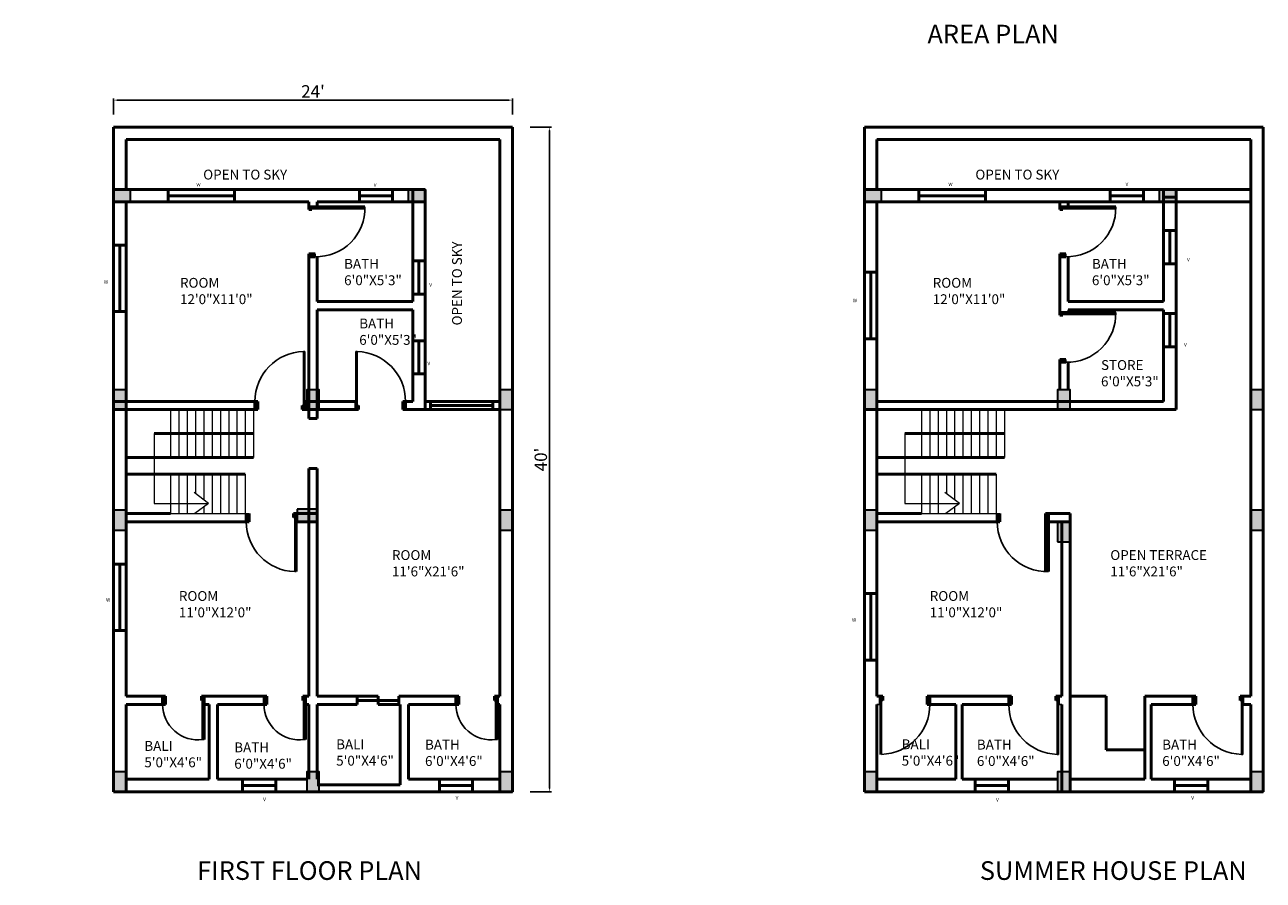
# Model space of a CAD drawing. Units: feet. Extents: x 1398 to 2768, y 682 to 1909.
# Tile 2 of 3: x 1874 to 2768, y 682 to 1300. Entities that reach past the tile are written whole.
import ezdxf

# ---------------------------------------------------------------- set-up
doc = ezdxf.new("R2010")
doc.units = ezdxf.units.FT
for name, color, linetype, lineweight in [('A-ANNO-DIMS', 2, 'Continuous', 18), ('A-ANNO-TEXT', 7, 'Continuous', 18), ('A-AREA-IDEN', 3, 'Continuous', 18), ('A-COLS', 7, 'Continuous', 35), ('A-DOOR', 4, 'Continuous', 25), ('A-FLOR-STRS', 3, 'Continuous', 18), ('A-WALL', 7, 'Continuous', 50), ('A-WALL-PATT', 8, 'Continuous', 13)]:
    doc.layers.add(name, color=color, linetype=linetype, lineweight=lineweight)
doc.styles.get("Standard").update_dxf_attribs({"font": 'arial.ttf'})
doc.dimstyles.new('ISO-25', dxfattribs={"dimtxt": 9, "dimasz": 2.5, "dimexe": 1.25, "dimexo": 0.625, "dimtad": 1, "dimdec": 1, "dimlunit": 3, "dimtxsty": 'Standard', "dimcen": 2.5, "dimadec": 0, "dimazin": 0, "dimtfac": 1, "dimtdec": 1, "dimtmove": 0, "dimatfit": 3, "dimfxl": 1, "dimarcsym": 0})

# ---------------------------------------------------------------- blocks, each defined once
blk = doc.blocks.new('*D3')
at = {"layer": 'A-ANNO-DIMS', "color": 0, "lineweight": -2, "transparency": 16777216}
for p, q in [((1937.94, 1235.32), (1937.94, 1246.88)), ((2223.44, 1245.63), (1940.44, 1245.63)), ((2225.94, 1235.32), (2225.94, 1246.88))]:
    blk.add_line(p, q, dxfattribs=at)
at = {"layer": 'A-ANNO-DIMS', "color": 0, "transparency": 16777216}
for points in [[(1940.44, 1246.04), (1940.44, 1245.21), (1937.94, 1245.63)], [(2223.44, 1246.04), (2223.44, 1245.21), (2225.94, 1245.63)]]:
    blk.add_solid(points, dxfattribs=at)
at = {"layer": 'Defpoints', "color": 0, "transparency": 16777216}
for p in [(1937.94, 1245.63), (1937.94, 1234.7), (2225.94, 1234.7)]:
    blk.add_point(p, dxfattribs=at)
at = {"layer": 'A-ANNO-DIMS', "color": 0, "transparency": 16777216, "insert": (2081.94, 1250.77), "char_height": 9, "attachment_point": 5}
blk.add_mtext("24'", dxfattribs=at)
blk = doc.blocks.new('*D4')
at = {"layer": 'A-ANNO-DIMS', "color": 0, "lineweight": -2, "transparency": 16777216}
for p, q in [((2238.9, 1226.08), (2254.12, 1226.08)), ((2252.87, 748.58), (2252.87, 1223.58)), ((2238.9, 746.08), (2254.12, 746.08))]:
    blk.add_line(p, q, dxfattribs=at)
at = {"layer": 'A-ANNO-DIMS', "color": 0, "transparency": 16777216}
for points in [[(2252.45, 1223.58), (2253.28, 1223.58), (2252.87, 1226.08)], [(2252.45, 748.58), (2253.28, 748.58), (2252.87, 746.08)]]:
    blk.add_solid(points, dxfattribs=at)
at = {"layer": 'Defpoints', "color": 0, "transparency": 16777216}
for p in [(2238.28, 1226.08), (2252.87, 1226.08), (2238.28, 746.08)]:
    blk.add_point(p, dxfattribs=at)
at = {"layer": 'A-ANNO-DIMS', "color": 0, "transparency": 16777216, "insert": (2247.65, 986.08), "char_height": 9, "attachment_point": 5, "rotation": 90}
blk.add_mtext("40'", dxfattribs=at)
blk = doc.blocks.new('DOOR-PLAN-900')
for p, q in [((1553.62, 938.08), (1552.62, 938.08)), ((1553.62, 899.08), (1553.62, 938.08)), ((1554.62, 935.08), (1554.62, 899.08)), ((1554.62, 899.08), (1553.62, 899.08))]:
    blk.add_line(p, q)
blk.add_arc((1554.63, 935.08), 36.01, 180, 268.38614)

msp = doc.modelspace()

# ---------------------------------------------------------------- hatches: boundary and pattern name
at = {"layer": 'A-WALL-PATT'}
h = msp.add_hatch(dxfattribs=at)
h.set_pattern_fill('BRASS', color=256, scale=0.02, style=0)
h.paths.add_polyline_path([(1425.8, 949.48), (1416.8, 949.48), (1416.8, 935.08), (1425.8, 935.08)])
h.paths.add_polyline_path([(1416.8, 1022.08), (1425.8, 1022.08), (1425.8, 1036.48), (1416.8, 1036.48)])
h.paths.add_polyline_path([(1565.3, 1036.48), (1556.3, 1036.48), (1556.3, 1022.08), (1565.3, 1022.08)])
h.paths.add_polyline_path([(1704.8, 1022.08), (1704.8, 1036.48), (1695.8, 1036.48), (1695.8, 1022.08)])
h.paths.add_polyline_path([(1695.8, 935.08), (1704.8, 935.08), (1704.8, 949.48), (1695.8, 949.48)])
h.paths.add_polyline_path([(1704.8, 746.08), (1704.8, 760.48), (1695.8, 760.48), (1695.8, 746.08)])
h.paths.add_polyline_path([(1565.3, 746.08), (1565.3, 760.48), (1556.3, 760.48), (1556.3, 746.08)])
h.paths.add_polyline_path([(1425.8, 746.08), (1425.8, 760.48), (1416.8, 760.48), (1416.8, 746.08)])
h.paths.add_polyline_path([(1428.8, 1181.08), (1416.8, 1181.08), (1416.8, 1172.09), (1428.8, 1172.09)])
h.paths.add_polyline_path([(1629.8, 1181.08), (1629.8, 1172.09), (1641.8, 1172.09), (1641.8, 1181.08)])
h.paths.add_polyline_path([(1937.94, 1022.08), (1946.94, 1022.08), (1946.94, 1036.48), (1937.94, 1036.48)])
h.paths.add_polyline_path([(1946.94, 949.48), (1937.94, 949.48), (1937.94, 935.08), (1946.94, 935.08)])
h.paths.add_polyline_path([(1946.94, 760.48), (1937.94, 760.48), (1937.94, 746.08), (1946.94, 746.08)])
h.paths.add_polyline_path([(2077.44, 746.08), (2086.44, 746.08), (2086.44, 760.48), (2077.44, 760.48)])
h.paths.add_polyline_path([(2070.54, 941.08), (2084.94, 941.08), (2084.94, 950.08), (2070.54, 950.08)])
h.paths.add_polyline_path([(2086.44, 1036.48), (2077.44, 1036.48), (2077.44, 1022.08), (2086.44, 1022.08)])
h.paths.add_polyline_path([(2162.94, 1172.09), (2162.94, 1181.08), (2150.94, 1181.08), (2150.94, 1172.09)])
h.paths.add_polyline_path([(1949.94, 1172.09), (1949.94, 1181.08), (1937.94, 1181.08), (1937.94, 1172.09)])
h.paths.add_polyline_path([(2216.94, 1022.08), (2225.94, 1022.08), (2225.94, 1036.48), (2216.94, 1036.48)])
h.paths.add_polyline_path([(2225.94, 935.08), (2225.94, 949.48), (2216.94, 949.48), (2216.94, 935.08)])
h.paths.add_polyline_path([(2216.94, 746.08), (2225.94, 746.08), (2225.94, 760.48), (2216.94, 760.48)])
h.paths.add_polyline_path([(2489.29, 760.48), (2480.29, 760.48), (2480.29, 746.08), (2489.29, 746.08)])
h.paths.add_polyline_path([(2628.79, 746.08), (2628.79, 760.48), (2619.79, 760.48), (2619.79, 746.08)])
h.paths.add_polyline_path([(2768.29, 760.48), (2759.29, 760.48), (2759.29, 746.08), (2768.29, 746.08)])
h.paths.add_polyline_path([(2768.29, 949.48), (2759.29, 949.48), (2759.29, 935.08), (2768.29, 935.08)])
h.paths.add_polyline_path([(2619.79, 926.68), (2628.79, 926.68), (2628.79, 941.08), (2619.79, 941.08)])
h.paths.add_polyline_path([(2489.29, 949.48), (2480.29, 949.48), (2480.29, 935.08), (2489.29, 935.08)])
h.paths.add_polyline_path([(2480.29, 1022.08), (2489.29, 1022.08), (2489.29, 1036.48), (2480.29, 1036.48)])
h.paths.add_polyline_path([(2628.79, 1036.48), (2619.79, 1036.48), (2619.79, 1022.08), (2628.79, 1022.08)])
h.paths.add_polyline_path([(2759.29, 1022.08), (2768.29, 1022.08), (2768.29, 1036.48), (2759.29, 1036.48)])
h.paths.add_polyline_path([(2693.29, 1172.09), (2705.29, 1172.09), (2705.29, 1181.08), (2693.29, 1181.08)])
h.paths.add_polyline_path([(2492.29, 1181.08), (2480.29, 1181.08), (2480.29, 1172.09), (2492.29, 1172.09)])

# ---------------------------------------------------------------- linework, layer by layer
at = {"layer": 'A-COLS'}
for points in [[(1937.94, 1181.08), (1949.94, 1181.08), (1949.94, 1172.09), (1937.94, 1172.09)], [(2150.94, 1181.08), (2162.94, 1181.08), (2162.94, 1172.09), (2150.94, 1172.09)], [(2480.29, 1181.08), (2492.29, 1181.08), (2492.29, 1172.09), (2480.29, 1172.09)], [(2693.29, 1181.08), (2705.29, 1181.08), (2705.29, 1172.09), (2693.29, 1172.09)], [(1937.94, 1022.08), (1946.94, 1022.08), (1946.94, 1036.48), (1937.94, 1036.48)], [(2077.44, 1022.08), (2086.44, 1022.08), (2086.44, 1036.48), (2077.44, 1036.48)], [(2216.94, 1022.08), (2225.94, 1022.08), (2225.94, 1036.48), (2216.94, 1036.48)], [(2480.29, 1022.08), (2489.29, 1022.08), (2489.29, 1036.48), (2480.29, 1036.48)], [(2619.79, 1022.08), (2628.79, 1022.08), (2628.79, 1036.48), (2619.79, 1036.48)], [(2759.29, 1022.08), (2768.29, 1022.08), (2768.29, 1036.48), (2759.29, 1036.48)], [(1937.94, 935.08), (1946.94, 935.08), (1946.94, 949.48), (1937.94, 949.48)], [(2070.54, 950.08), (2070.54, 941.08), (2084.94, 941.08), (2084.94, 950.08)], [(2216.94, 935.08), (2225.94, 935.08), (2225.94, 949.48), (2216.94, 949.48)], [(2480.29, 935.08), (2489.29, 935.08), (2489.29, 949.48), (2480.29, 949.48)], [(2759.29, 935.08), (2768.29, 935.08), (2768.29, 949.48), (2759.29, 949.48)], [(2619.79, 926.68), (2628.79, 926.68), (2628.79, 941.08), (2619.79, 941.08)], [(1937.94, 746.08), (1946.94, 746.08), (1946.94, 760.48), (1937.94, 760.48)], [(2077.44, 746.08), (2086.44, 746.08), (2086.44, 760.48), (2077.44, 760.48)], [(2216.94, 746.08), (2225.94, 746.08), (2225.94, 760.48), (2216.94, 760.48)], [(2480.29, 746.08), (2489.29, 746.08), (2489.29, 760.48), (2480.29, 760.48)], [(2619.79, 746.08), (2628.79, 746.08), (2628.79, 760.48), (2619.79, 760.48)], [(2759.29, 746.08), (2768.29, 746.08), (2768.29, 760.48), (2759.29, 760.48)]]:
    msp.add_lwpolyline(points, close=True, dxfattribs=at)
at = {"layer": 'A-DOOR'}
for p, q in [((2081.19, 1167.56), (2081.19, 1166.58)), ((2623.54, 1167.55), (2623.54, 1166.56)), ((2083.44, 1134.56), (2083.44, 1132.56)), ((2625.79, 1134.55), (2625.79, 1132.55)), ((2627.29, 1094.07), (2627.29, 1092.31)), ((2623.54, 1091.31), (2623.54, 1090.33)), ((2625.79, 1058.31), (2625.79, 1056.31)), ((2068.76, 944.08), (2067.76, 944.08)), ((2068.76, 905.08), (2068.76, 944.08)), ((2069.76, 905.08), (2068.76, 905.08)), ((2489.29, 809.08), (2491.54, 809.08)), ((2491.54, 809.08), (2491.54, 773.08)), ((2492.54, 773.08), (2492.54, 812.08)), ((2492.54, 812.08), (2493.54, 812.08)), ((2619.49, 809.08), (2622.79, 809.08)), ((2003.32, 783.88), (2002.32, 783.88)), ((2076.64, 783.88), (2075.64, 783.88)), ((2215.16, 783.88), (2214.16, 783.88))]:
    msp.add_line(p, q, dxfattribs=at)
for centre, radius, start, end in [((2084.43, 1167.56), 35.01, 268.38614, 1.6366), ((2626.78, 1167.55), 35.01, 268.38614, 1.6366), ((2626.78, 1091.31), 35.01, 268.38614, 1.6366), ((2069.78, 941.08), 36.01, 180, 268.38614), ((2612.12, 941.08), 36.01, 180, 271.56839), ((1998.77, 809.08), 25.45, 180, 278.02097), ((2072.09, 809.08), 25.45, 180, 278.02097), ((2210.61, 809.08), 25.45, 180, 278.02097), ((2491.52, 809.08), 36.01, 271.61386, 360)]:
    msp.add_arc(centre, radius, start, end, dxfattribs=at)
at = {"layer": 'A-FLOR-STRS'}
for p, q in [((1979.05, 1022.08), (1979.05, 987.58)), ((1985.05, 1022.08), (1985.05, 987.58)), ((1991.05, 1022.08), (1991.05, 987.58)), ((1997.05, 1022.08), (1997.05, 987.58)), ((2003.05, 1022.08), (2003.05, 987.58)), ((2009.05, 1022.08), (2009.05, 987.58)), ((2015.05, 1022.08), (2015.05, 987.58)), ((2021.05, 1022.08), (2021.05, 987.58)), ((2027.05, 1022.08), (2027.05, 987.58)), ((2033.05, 1022.08), (2033.05, 987.58)), ((2039.05, 1022.08), (2039.05, 987.58)), ((2521.4, 1022.08), (2521.4, 987.58)), ((2527.4, 1022.08), (2527.4, 987.58)), ((2533.4, 1022.08), (2533.4, 987.58)), ((2539.4, 1022.08), (2539.4, 987.58)), ((2545.4, 1022.08), (2545.4, 987.58)), ((2551.4, 1022.08), (2551.4, 987.58)), ((2557.4, 1022.08), (2557.4, 987.58)), ((2563.4, 1022.08), (2563.4, 987.58)), ((2569.4, 1022.08), (2569.4, 987.58)), ((2575.4, 1022.08), (2575.4, 987.58)), ((2581.4, 1022.08), (2581.4, 987.58)), ((1967.14, 1004.83), (1967.14, 954.35)), ((2509.48, 1004.83), (2509.48, 954.35)), ((1979.05, 975.58), (1979.05, 947.08)), ((1985.05, 975.58), (1985.05, 947.08)), ((1991.05, 975.58), (1991.05, 947.08)), ((1997.05, 975.58), (1997.05, 961.37)), ((2003.05, 975.58), (2003.05, 956.91)), ((2009.05, 975.58), (2009.05, 947.08)), ((2015.05, 975.58), (2015.05, 947.08)), ((2021.05, 975.58), (2021.05, 947.08)), ((2027.05, 975.58), (2027.05, 947.08)), ((2033.05, 975.58), (2033.05, 947.08)), ((2521.4, 975.58), (2521.4, 947.08)), ((2527.4, 975.58), (2527.4, 947.08)), ((2533.4, 975.58), (2533.4, 947.08)), ((2539.4, 975.58), (2539.4, 961.37)), ((2545.4, 975.58), (2545.4, 956.91)), ((2551.4, 975.58), (2551.4, 947.08)), ((2557.4, 975.58), (2557.4, 947.08)), ((2563.4, 975.58), (2563.4, 947.08)), ((2569.4, 975.58), (2569.4, 947.08)), ((2575.4, 975.58), (2575.4, 947.08)), ((2006.5, 954.35), (1996.03, 962.13)), ((2548.85, 954.35), (2538.38, 962.13)), ((1967.14, 954.35), (2006.5, 954.35)), ((2006.5, 954.35), (1996.71, 947.08)), ((2003.05, 951.79), (2003.05, 947.08)), ((2509.48, 954.35), (2548.85, 954.35)), ((2548.85, 954.35), (2539.06, 947.08)), ((2545.4, 951.79), (2545.4, 947.08)), ((1979.05, 947.08), (2035.76, 947.08)), ((2521.4, 947.08), (2578.11, 947.08))]:
    msp.add_line(p, q, dxfattribs=at)
at = {"layer": 'A-WALL'}
for p, q in [((2225.94, 1226.08), (1937.94, 1226.08)), ((1937.94, 1226.08), (1937.94, 746.08)), ((2225.94, 746.08), (2225.94, 1226.08)), ((2768.29, 1226.08), (2480.29, 1226.08)), ((2480.29, 1226.08), (2480.29, 746.08)), ((2768.29, 746.08), (2768.29, 1226.08)), ((1946.94, 1217.08), (1946.94, 1181.08)), ((2216.94, 1217.08), (1946.94, 1217.08)), ((2216.94, 815.08), (2216.94, 1217.08)), ((2759.29, 1217.08), (2489.29, 1217.08)), ((2489.29, 1217.08), (2489.29, 1181.08)), ((2759.29, 815.08), (2759.29, 1217.08)), ((1937.94, 1181.08), (2162.94, 1181.08)), ((1977.22, 1181.08), (1977.22, 1172.08)), ((2025.22, 1181.08), (2025.22, 1172.08)), ((2115.43, 1181.08), (2115.43, 1172.08)), ((2139.43, 1181.08), (2139.43, 1172.08)), ((2153.94, 1181.08), (2153.94, 1100.08)), ((2162.94, 1181.08), (2162.94, 1022.08)), ((2480.29, 1181.08), (2759.29, 1181.08)), ((2519.57, 1181.07), (2519.57, 1172.07)), ((2567.57, 1181.07), (2567.57, 1172.07)), ((2657.77, 1181.07), (2657.77, 1172.07)), ((2681.77, 1181.07), (2681.77, 1172.07)), ((2696.29, 1181.08), (2696.29, 1100.07)), ((2705.29, 1181.08), (2705.29, 1022.08)), ((1937.94, 1172.08), (2078.94, 1172.08)), ((1946.94, 1172.09), (1946.94, 815.08)), ((1946.94, 1172.09), (1946.94, 1036.48)), ((1977.22, 1176.58), (2025.22, 1176.58)), ((2078.94, 1172.09), (2078.94, 1166.58)), ((2084.94, 1172.09), (2084.94, 1167.56)), ((2084.94, 1172.08), (2162.94, 1172.08)), ((2115.43, 1176.58), (2139.43, 1176.58)), ((2480.29, 1172.08), (2759.29, 1172.08)), ((2480.29, 1172.07), (2621.29, 1172.07)), ((2489.29, 1172.09), (2489.29, 815.08)), ((2519.57, 1176.57), (2567.57, 1176.57)), ((2621.29, 1172.08), (2621.29, 1166.56)), ((2627.29, 1172.08), (2627.29, 1167.55)), ((2657.77, 1176.57), (2681.77, 1176.57)), ((2705.29, 1175.43), (2696.29, 1175.43)), ((2083.44, 1168.56), (2078.94, 1168.56)), ((2081.19, 1166.58), (2078.94, 1166.58)), ((2119.44, 1167.56), (2081.19, 1167.56)), ((2083.44, 1168.56), (2119.44, 1168.56)), ((2625.79, 1168.55), (2621.29, 1168.55)), ((2623.54, 1166.56), (2621.29, 1166.56)), ((2661.79, 1167.55), (2623.54, 1167.55)), ((2625.79, 1168.55), (2661.79, 1168.55)), ((2705.29, 1151.43), (2696.29, 1151.43)), ((2700.79, 1151.43), (2700.79, 1127.43)), ((1946.94, 1140.96), (1937.94, 1140.96)), ((1942.44, 1140.96), (1942.44, 1092.96)), ((2083.44, 1134.56), (2078.94, 1134.56)), ((2078.94, 1134.56), (2078.94, 1036.48)), ((2083.44, 1132.56), (2078.94, 1132.56)), ((2084.94, 1132.55), (2084.94, 1100.08)), ((2162.94, 1129.53), (2153.94, 1129.53)), ((2158.44, 1129.53), (2158.44, 1105.53)), ((2621.29, 1134.55), (2621.29, 1090.33)), ((2625.79, 1134.55), (2621.29, 1134.55)), ((2625.79, 1132.55), (2621.29, 1132.55)), ((2627.29, 1132.54), (2627.29, 1100.07)), ((2705.29, 1127.43), (2696.29, 1127.43)), ((2489.29, 1121.3), (2480.29, 1121.3)), ((2484.79, 1121.3), (2484.79, 1073.3)), ((2162.94, 1105.53), (2153.94, 1105.53)), ((1946.94, 1092.96), (1937.94, 1092.96)), ((2084.94, 1100.08), (2153.94, 1100.08)), ((2084.94, 1094.08), (2153.94, 1094.08)), ((2084.94, 1094.08), (2084.94, 1036.48)), ((2153.94, 1094.08), (2153.94, 1028.08)), ((2625.79, 1092.31), (2621.29, 1092.31)), ((2625.79, 1092.31), (2661.79, 1092.31)), ((2627.29, 1100.07), (2696.29, 1100.07)), ((2627.29, 1094.07), (2696.29, 1094.07)), ((2696.29, 1094.07), (2696.29, 1028.08)), ((2705.29, 1091.43), (2696.29, 1091.43)), ((2700.79, 1091.43), (2700.79, 1067.43)), ((2623.54, 1090.33), (2621.29, 1090.33)), ((2661.79, 1091.31), (2623.54, 1091.31)), ((2162.94, 1071.89), (2153.94, 1071.89)), ((2158.44, 1071.89), (2158.44, 1047.89)), ((2489.29, 1073.3), (2480.29, 1073.3)), ((2705.29, 1067.43), (2696.29, 1067.43)), ((2625.79, 1058.31), (2621.29, 1058.31)), ((2621.29, 1058.31), (2621.29, 1036.47)), ((2625.79, 1056.31), (2621.29, 1056.31)), ((2627.29, 1056.3), (2627.29, 1036.47)), ((2162.94, 1047.89), (2153.94, 1047.89)), ((2078.94, 1015.65), (2078.94, 1045.77)), ((2084.94, 1015.65), (2084.94, 1045.77)), ((1937.94, 1028.08), (2042, 1028.08)), ((1937.94, 1022.08), (2042, 1022.08)), ((1946.94, 1022.08), (1946.94, 941.08)), ((2040, 1028.08), (2040, 1022.08)), ((2040, 1022.08), (2040, 1028.08)), ((2042, 1022.08), (2042, 1028.08)), ((2074, 1025.08), (2074, 1022.08)), ((2074, 1022.08), (2114.78, 1022.08)), ((2076, 1028.08), (2076, 1022.08)), ((2076, 1028.08), (2112.78, 1028.08)), ((2112.78, 1028.08), (2112.78, 1022.08)), ((2114.78, 1025.08), (2114.78, 1022.08)), ((2146.78, 1028.08), (2153.94, 1028.08)), ((2146.78, 1022.08), (2146.78, 1028.08)), ((2146.78, 1022.08), (2216.94, 1022.08)), ((2148.78, 1028.08), (2148.78, 1022.08)), ((2148.78, 1022.08), (2148.78, 1028.08)), ((2162.94, 1028.08), (2216.94, 1028.08)), ((2166.78, 1028.08), (2166.78, 1022.08)), ((2166.78, 1025.08), (2210.83, 1025.08)), ((2210.83, 1025.08), (2211.95, 1025.08)), ((2211.95, 1028.08), (2211.95, 1022.08)), ((2480.29, 1022.08), (2584.35, 1022.08)), ((2696.29, 1028.08), (2489.29, 1028.08)), ((2705.29, 1022.08), (2489.29, 1022.08)), ((2084.94, 1015.65), (2078.94, 1015.65)), ((2039.05, 1004.83), (1967.14, 1004.83)), ((2581.4, 1004.83), (2509.48, 1004.83)), ((2039.05, 987.58), (1946.94, 987.58)), ((2581.4, 987.58), (2489.29, 987.58)), ((2033.05, 975.58), (1946.94, 975.58)), ((2078.94, 941.08), (2078.94, 979.65)), ((2084.94, 979.65), (2078.94, 979.65)), ((2084.94, 941.08), (2084.94, 979.65)), ((2575.4, 975.58), (2489.29, 975.58)), ((1979.05, 947.08), (1946.94, 947.08)), ((1979.05, 941.08), (1946.94, 941.08)), ((1979.05, 941.08), (2035.76, 941.08)), ((2033.76, 947.08), (2033.76, 941.08)), ((2035.76, 947.08), (2035.76, 941.08)), ((2067.76, 944.08), (2067.76, 947.08)), ((2067.76, 947.08), (2069.76, 947.08)), ((2067.76, 947.08), (2084.94, 947.08)), ((2068.76, 941.08), (2084.94, 941.08)), ((2069.76, 947.08), (2069.76, 905.08)), ((2078.94, 941.08), (2078.94, 815.08)), ((2084.94, 941.08), (2084.94, 815.08)), ((2521.4, 947.08), (2489.29, 947.08)), ((2521.4, 941.08), (2489.29, 941.08)), ((2521.4, 941.08), (2578.11, 941.08)), ((2576.11, 947.08), (2576.11, 941.08)), ((2578.11, 947.08), (2578.11, 941.08)), ((2611.11, 947.08), (2628.79, 947.08)), ((2611.11, 905.08), (2611.11, 947.08)), ((2613.11, 905.08), (2613.11, 947.08)), ((2628.79, 941.08), (2613.11, 941.08)), ((2622.79, 941.08), (2622.79, 815.08)), ((2628.79, 947.08), (2628.79, 815.08)), ((1946.94, 910.47), (1937.94, 910.47)), ((1942.44, 910.47), (1942.44, 862.47)), ((2489.29, 889.19), (2480.29, 889.19)), ((2484.79, 889.19), (2484.79, 841.19)), ((1946.94, 862.47), (1937.94, 862.47)), ((2489.29, 841.19), (2480.29, 841.19)), ((1946.94, 815.08), (1975.32, 815.08)), ((1973.32, 815.08), (1973.32, 809.08)), ((1975.32, 815.08), (1975.32, 809.08)), ((2001.32, 815.08), (2002.13, 815.08)), ((2001.32, 812.08), (2001.32, 815.08)), ((2001.32, 815.08), (2048.64, 815.08)), ((2003.32, 815.08), (2003.32, 809.08)), ((2046.64, 815.08), (2046.64, 809.08)), ((2048.64, 815.08), (2048.64, 809.08)), ((2074.64, 812.08), (2074.64, 815.08)), ((2074.64, 815.08), (2078.94, 815.08)), ((2076.64, 815.08), (2076.64, 809.08)), ((2084.94, 815.08), (2113.9, 815.08)), ((2113.9, 815.08), (2113.9, 809.08)), ((2128.9, 815.08), (2113.9, 815.08)), ((2128.9, 812.08), (2128.9, 815.08)), ((2143.9, 815.08), (2143.9, 809.08)), ((2143.9, 815.08), (2187.16, 815.08)), ((2185.16, 815.08), (2185.16, 809.08)), ((2187.16, 815.08), (2187.16, 809.08)), ((2213.16, 812.08), (2213.16, 815.08)), ((2213.16, 815.08), (2216.94, 815.08)), ((2215.16, 815.08), (2215.16, 809.08)), ((2489.29, 815.08), (2493.54, 815.08)), ((2491.54, 815.08), (2491.54, 809.08)), ((2493.54, 812.08), (2493.54, 815.08)), ((2525.54, 815.08), (2525.54, 809.08)), ((2525.54, 815.08), (2586.49, 815.08)), ((2527.54, 815.08), (2527.54, 809.08)), ((2584.49, 815.08), (2584.49, 809.08)), ((2586.49, 815.08), (2586.49, 809.08)), ((2618.49, 812.08), (2618.49, 815.08)), ((2618.49, 815.08), (2622.79, 815.08)), ((2620.49, 815.08), (2620.49, 809.08)), ((2628.79, 815.08), (2654.96, 815.08)), ((2628.79, 815.08), (2628.79, 746.08)), ((2654.96, 815.08), (2654.96, 776.37)), ((2682.79, 755.08), (2682.79, 815.08)), ((2682.79, 815.08), (2719.54, 815.08)), ((2717.54, 815.08), (2717.54, 809.08)), ((2719.54, 815.08), (2719.54, 809.08)), ((2751.54, 812.08), (2751.54, 815.08)), ((2751.54, 815.08), (2759.29, 815.08)), ((2753.54, 815.08), (2753.54, 809.08)), ((1946.94, 809.08), (1975.32, 809.08)), ((1946.94, 809.08), (1946.94, 746.08)), ((2002.32, 812.08), (2001.32, 812.08)), ((2002.32, 783.88), (2002.32, 812.08)), ((2003.32, 809.08), (2003.32, 783.88)), ((2003.32, 809.08), (2006.94, 809.08)), ((2006.94, 809.08), (2006.94, 755.08)), ((2012.94, 809.08), (2012.94, 755.08)), ((2012.94, 809.08), (2048.64, 809.08)), ((2075.64, 812.08), (2074.64, 812.08)), ((2075.64, 783.88), (2075.64, 812.08)), ((2076.64, 809.08), (2076.64, 783.88)), ((2076.64, 809.08), (2078.94, 809.08)), ((2078.94, 809.08), (2078.94, 755.08)), ((2084.94, 809.08), (2113.9, 809.08)), ((2084.94, 809.08), (2084.94, 755.08)), ((2143.9, 812.08), (2113.9, 812.08)), ((2128.9, 812.08), (2128.9, 809.08)), ((2128.9, 809.08), (2143.9, 809.08)), ((2142.9, 812.08), (2141.9, 812.08)), ((2143.9, 809.08), (2144.94, 809.08)), ((2144.94, 809.08), (2144.94, 755.08)), ((2150.94, 809.08), (2150.94, 755.08)), ((2150.94, 809.08), (2187.16, 809.08)), ((2214.16, 812.08), (2213.16, 812.08)), ((2214.16, 783.88), (2214.16, 812.08)), ((2215.16, 809.08), (2215.16, 783.88)), ((2215.16, 809.08), (2216.94, 809.08)), ((2216.94, 746.08), (2216.94, 809.08)), ((2489.29, 809.08), (2489.29, 746.08)), ((2525.54, 809.08), (2546.29, 809.08)), ((2546.29, 809.08), (2546.29, 755.08)), ((2550.79, 809.08), (2550.79, 755.08)), ((2550.79, 809.08), (2586.49, 809.08)), ((2622.79, 809.08), (2622.79, 746.08)), ((2687.29, 755.08), (2687.29, 809.08)), ((2687.29, 809.08), (2719.54, 809.08)), ((2753.54, 809.08), (2759.29, 809.08)), ((2759.29, 746.08), (2759.29, 809.08)), ((2654.96, 776.37), (2682.79, 776.37)), ((1946.94, 755.08), (2006.94, 755.08)), ((2012.94, 755.08), (2077.44, 755.08)), ((2031.02, 755.08), (2031.02, 746.08)), ((2055.02, 755.08), (2055.02, 746.08)), ((2086.44, 755.08), (2084.94, 755.08)), ((2086.44, 753.08), (2084.94, 753.08)), ((2144.94, 755.08), (2144.94, 751.08)), ((2150.94, 755.08), (2216.94, 755.08)), ((2173.25, 755.08), (2173.25, 746.08)), ((2197.25, 755.08), (2197.25, 746.08)), ((2489.29, 755.08), (2546.29, 755.08)), ((2550.79, 755.08), (2619.79, 755.08)), ((2560.19, 755.08), (2560.19, 746.08)), ((2584.19, 755.08), (2584.19, 746.08)), ((2628.79, 755.08), (2682.79, 755.08)), ((2687.29, 755.08), (2759.29, 755.08)), ((2704.19, 755.08), (2704.19, 746.08)), ((2728.19, 755.08), (2728.19, 746.08)), ((1937.94, 746.08), (2225.94, 746.08)), ((2031.02, 750.58), (2055.02, 750.58)), ((2144.94, 751.08), (2084.94, 751.08)), ((2173.25, 750.58), (2197.25, 750.58)), ((2480.29, 746.08), (2768.29, 746.08)), ((2560.19, 750.58), (2584.19, 750.58)), ((2704.19, 750.58), (2727.23, 750.58)), ((2727.23, 750.58), (2728.19, 750.58))]:
    msp.add_line(p, q, dxfattribs=at)

# ---------------------------------------------------------------- block references
at = {"layer": 'A-DOOR', "extrusion": (0, 0, -1), "zscale": -1, "rotation": 180}
msp.add_blockref('DOOR-PLAN-900', (-521.38, 1963.16), dxfattribs=at)
at = {"layer": 'A-DOOR', "rotation": 180}
msp.add_blockref('DOOR-PLAN-900', (3667.4, 1963.16), dxfattribs=at)
at = {"layer": 'A-DOOR'}
for p in [(1065.87, -126), (1198.92, -126)]:
    msp.add_blockref('DOOR-PLAN-900', p, dxfattribs=at)

# ---------------------------------------------------------------- texts
at = {"layer": 'A-ANNO-TEXT', "attachment_point": 1}
for s, width, gutter_width, insert, char_height in [('AREA PLAN', 449.1316, 67.3, (2525.76, 1300.06), 13.459), ('W', 29.3663, 12.5, (1997.74, 1185.75), 2.5), ('V', 29.3663, 12.5, (2125.84, 1185.56), 2.5), ('W', 29.3663, 12.5, (2540.89, 1186.04), 2.5), ('V', 29.3663, 12.5, (2668.88, 1186.09), 2.5), ('V', 29.3663, 12.5, (2713.27, 1131.72), 2.5), ('W', 29.3663, 12.5, (1930.9, 1115.46), 2.5), ('V', 29.3663, 12.5, (2165.93, 1113.43), 2.5), ('W', 29.3663, 12.5, (2471.85, 1102.18), 2.5), ('V', 29.3663, 12.5, (2711.12, 1070.17), 2.5), ('V', 29.3663, 12.5, (2164.62, 1056.7), 2.5), ('W', 29.3663, 12.5, (1932.52, 885.96), 2.5), ('W', 29.3663, 12.5, (2471.3, 871.49), 2.5), ('V', 29.3663, 12.5, (2184.97, 742.99), 2.5), ('V', 29.3663, 12.5, (2716.31, 742.95), 2.5), ('V', 29.3663, 12.5, (2045.93, 741.73), 2.5), ('V', 29.3663, 12.5, (2575.35, 741.53), 2.5), ('FIRST FLOOR PLAN ', 449.1316, 67.3, (1998.29, 695.89), 13.4591), ('SUMMER HOUSE PLAN', 449.1316, 67.3, (2563.6, 695.89), 13.4591)]:
    msp.add_mtext_dynamic_manual_height_columns(s, width=width, gutter_width=gutter_width, heights=[0], dxfattribs=dict(at, insert=insert, char_height=char_height))
at = {"layer": 'A-AREA-IDEN', "attachment_point": 1}
for s, insert, char_height in [('OPEN TO SKY', (2002.64, 1195.41), 7.1088), ('OPEN TO SKY', (2560.37, 1195.41), 7.1088), ('BATH\\P6\'0"X5\'3"', (2104.43, 1130.94), 7.109), ('BATH\\P6\'0"X5\'3"', (2644.55, 1130.94), 7.109), ('ROOM\\P12\'0"X11\'0"', (1985.88, 1117.25), 7.1088), ('ROOM\\P12\'0"X11\'0"', (2529.57, 1117.25), 7.1088), ('BATH\\P6\'0"X5\'3"', (2115.33, 1087.86), 7.109), ('STORE\\P6\'0"X5\'3"', (2651.12, 1057.87), 7.109), ('ROOM\\P11\'6"X21\'6"', (2138.97, 920.61), 7.1088), ('OPEN TERRACE \\P11\'6"X21\'6"', (2657.84, 920.61), 7.1088), ('ROOM\\P11\'0"X12\'0"', (1985.07, 891.04), 7.1088), ('ROOM\\P11\'0"X12\'0"', (2527.42, 891.04), 7.1088), ('BALI\\P5\'0"X4\'6"', (1960.13, 782.73), 7.109), ('BATH\\P6\'0"X4\'6"', (2025.07, 781.71), 7.109), ('BALI\\P5\'0"X4\'6"', (2098.7, 783.91), 7.109), ('BATH\\P6\'0"X4\'6"', (2162.86, 783.69), 7.109), ('BALI\\P5\'0"X4\'6"', (2507.14, 783.91), 7.109), ('BATH\\P6\'0"X4\'6"', (2561.47, 783.69), 7.109), ('BATH\\P6\'0"X4\'6"', (2695.32, 783.69), 7.109)]:
    msp.add_mtext_dynamic_manual_height_columns(s, width=237.2218, gutter_width=35.54, heights=[0], dxfattribs=dict(at, insert=insert, char_height=char_height))
at = {"layer": 'A-AREA-IDEN', "insert": (2182.41, 1082.92), "char_height": 7.1088, "attachment_point": 1, "rotation": 90}
msp.add_mtext_dynamic_manual_height_columns('OPEN TO SKY', width=237.2218, gutter_width=35.54, heights=[0], dxfattribs=at)

# ---------------------------------------------------------------- dimensions: what is measured, and where the dimension line sits
at = {"layer": 'A-ANNO-DIMS'}
dim = msp.add_linear_dim(base=(1937.94, 1245.63), p1=(2225.94, 1234.7), p2=(1937.94, 1234.7), dimstyle='ISO-25', override={"dimclrd": 0, "dimclre": 0, "dimclrt": 0}, dxfattribs=at)
dim.commit()
dim.dimension.update_dxf_attribs({"geometry": '*D3', "text_midpoint": (2081.94, 1250.77)})
dim = msp.add_linear_dim(base=(2252.87, 1226.08), p1=(2238.28, 746.08), p2=(2238.28, 1226.08), angle=90, dimstyle='ISO-25', override={"dimclrd": 0, "dimclre": 0, "dimclrt": 0}, dxfattribs=at)
dim.commit()
dim.dimension.update_dxf_attribs({"geometry": '*D4', "text_midpoint": (2247.65, 986.08)})

doc.saveas('drawing.dxf')
